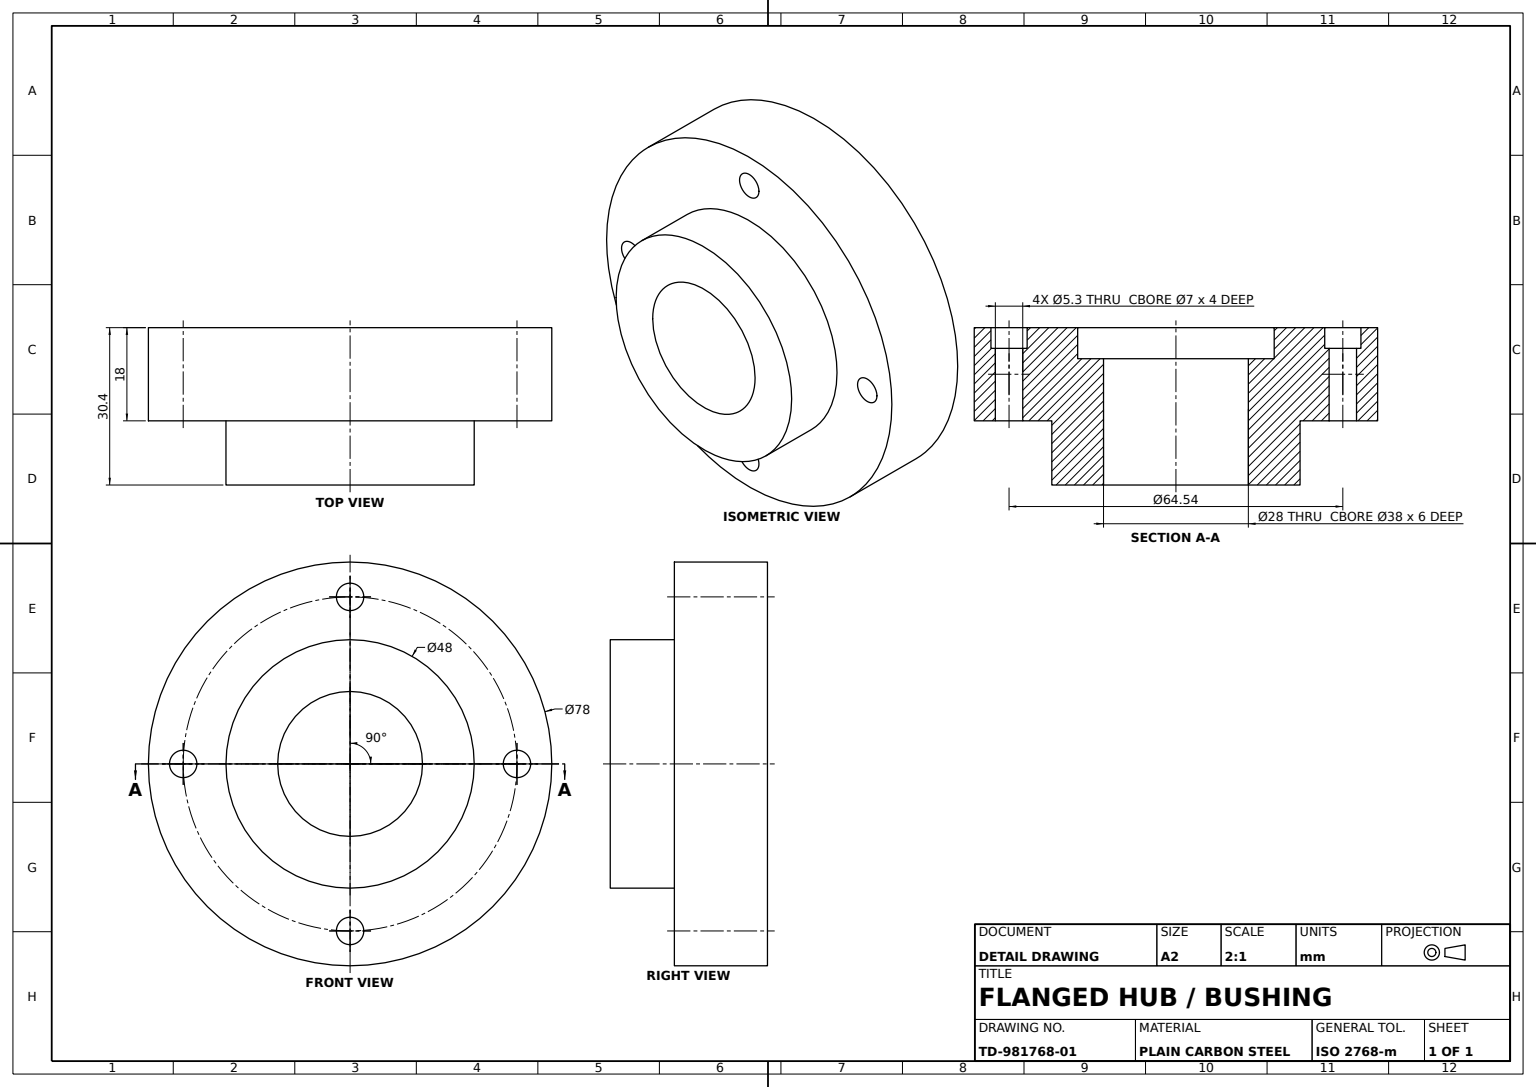
from build123d import *

# Parameters (mm, degrees)
HUB_PROFILE_SKETCH_W        = 5
HUB_PROFILE_SKETCH_H        = 20
HUB_PROFILE_SKETCH_W_2      = 4
MOUNTING_HOLES_SKETCH_R     = 14
MOUNTING_HOLES_SKETCH_R_2   = 2.65
MOUNTING_HOLES_4X_5_3_DEPTH = 317
SLOT_SKETCH_R               = 3.5
SLOT_7MM_X_4_DEEP_DEPTH     = 4
RECESS_SKETCH_R             = 19
RECESS_38_X_6_DEEP_DEPTH    = 6


with BuildPart() as part:
    # Hub Profile Sketch → Flanged Hub Body (revolve)
    with BuildSketch(Plane.XY, mode=Mode.PRIVATE) as flanged_hub_body_sk:
        with BuildLine():
            Line((-5, -19), (0, -19))
            Line((0, -19), (4.6, -19))
            ThreePointArc((4.6, -19), (6.014213562, -18.414213562), (6.6, -17))
            Line((6.6, -17), (6.6, 0))
            Line((6.6, 0), (-9, 0))
            Line((-9, 0), (-9, -19))
            Line((-9, -19), (-5, -19))
        make_face()
        with BuildLine():
            Line((9, -39), (9, -24))
            Line((9, -24), (21.4, -24))
            Line((21.4, -24), (21.4, 0))
            Line((21.4, 0), (6.6, 0))
            Line((6.6, 0), (6.6, -17))
            ThreePointArc((6.6, -17), (6.014213562, -18.414213562), (4.6, -19))
            Line((4.6, -19), (0, -19))
            Line((0, -19), (0, -39))
            Line((0, -39), (9, -39))
        make_face()
        with Locations((-2.5, -29)):
            Rectangle(HUB_PROFILE_SKETCH_W, HUB_PROFILE_SKETCH_H)
        with Locations((-7, -29)):
            Rectangle(HUB_PROFILE_SKETCH_W_2, HUB_PROFILE_SKETCH_H)
    revolve(flanged_hub_body_sk.sketch.rotate(Axis((6.6, 0, 0), (1, 0, 0)), 270), axis=Axis((6.6, 0, 0), (1, 0, 0)))

    # Mounting Holes Sketch → Mounting Holes 4xØ5.3 (cut)
    with BuildSketch(Plane(origin=(21.4, 0, 0), x_dir=(0, 0, -1), z_dir=(1, 0, 0))):
        Circle(MOUNTING_HOLES_SKETCH_R)
        with Locations(Location((0, 32.26943336, 0), (0, 0, 180))):
            Circle(MOUNTING_HOLES_SKETCH_R_2)
        with Locations(Location((32.26943336, 0, 0), (0, 0, 180))):
            Circle(MOUNTING_HOLES_SKETCH_R_2)
        with Locations(Location((0, -32.26943336, 0), (0, 0, 180))):
            Circle(MOUNTING_HOLES_SKETCH_R_2)
        with Locations(Location((-32.26943336, 0, 0), (0, 0, 180))):
            Circle(MOUNTING_HOLES_SKETCH_R_2)
    extrude(amount=-MOUNTING_HOLES_4X_5_3_DEPTH, mode=Mode.SUBTRACT)

    # Slot Sketch → Slot 7mm x 4 Deep (cut)
    with BuildSketch(Plane.ZY.offset(9)):
        with Locations((0, 32.26943336)):
            Circle(SLOT_SKETCH_R)
        with Locations((-32.26943336, 0)):
            Circle(SLOT_SKETCH_R)
        with Locations((0, -32.26943336)):
            Circle(SLOT_SKETCH_R)
        with Locations((32.26943336, 0)):
            Circle(SLOT_SKETCH_R)
    extrude(amount=-SLOT_7MM_X_4_DEEP_DEPTH, mode=Mode.SUBTRACT)

    # Recess Sketch → Recess Ø38 x 6 Deep (cut)
    with BuildSketch(Plane.ZY.offset(9)):
        Circle(RECESS_SKETCH_R)
    extrude(amount=-RECESS_38_X_6_DEEP_DEPTH, mode=Mode.SUBTRACT)


solid = part.part
